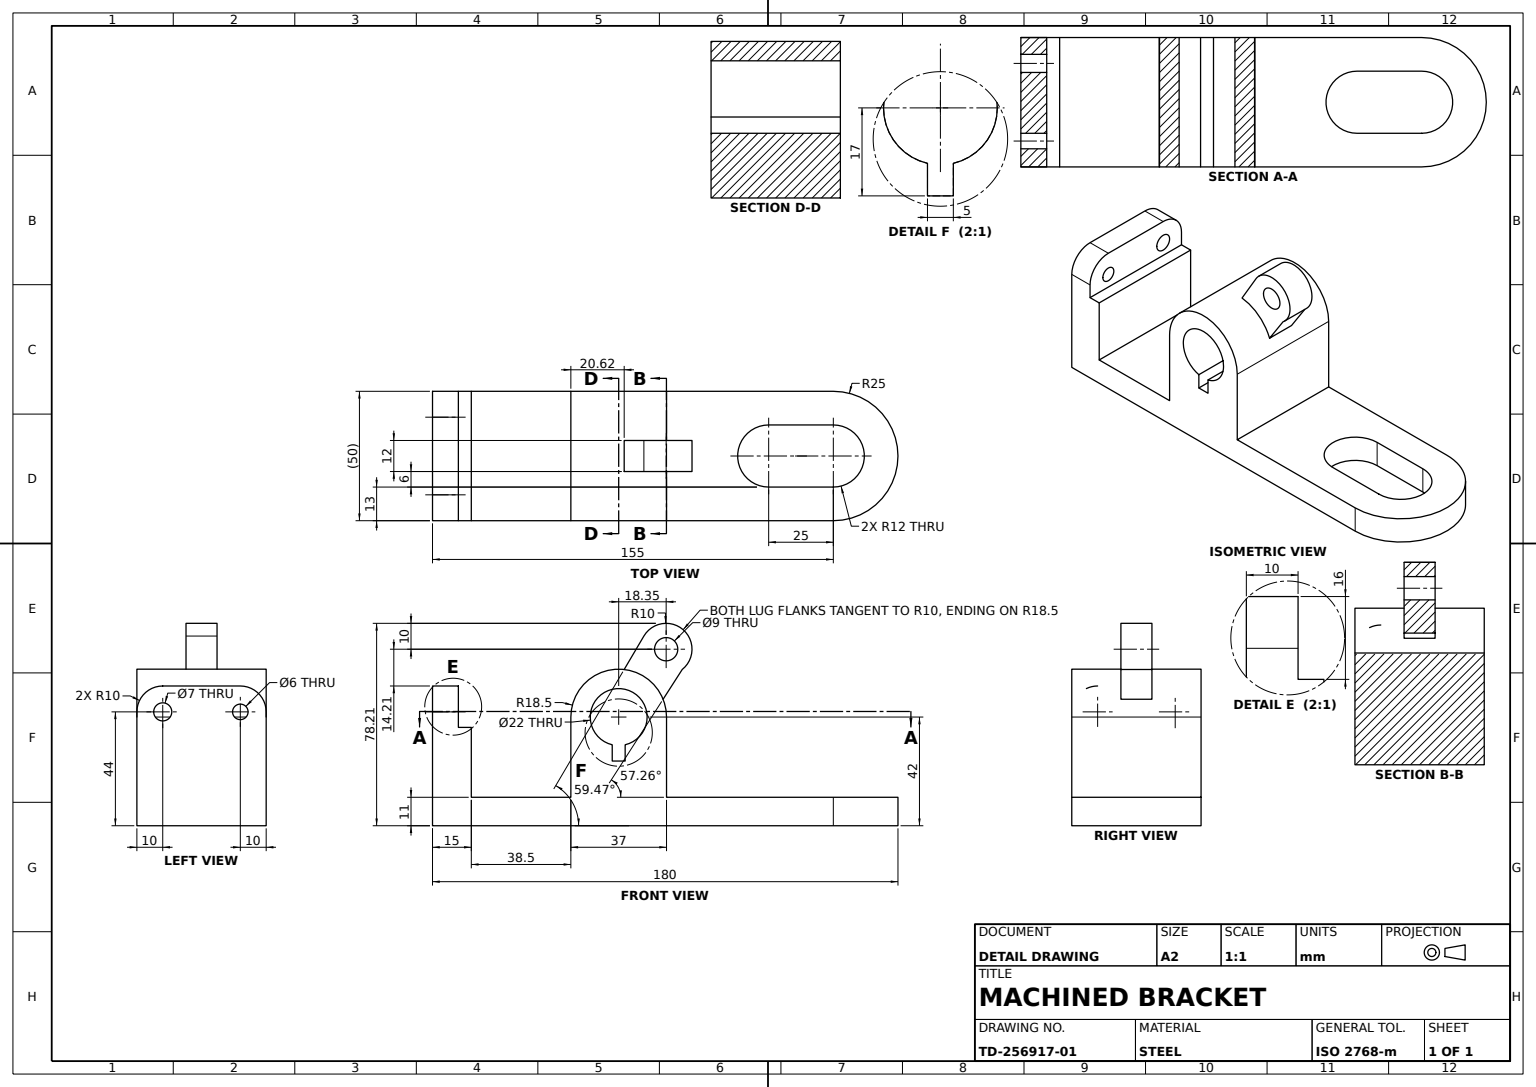
from build123d import *

# Parameters (mm, degrees)
BASE_PLATE_11MM_DEPTH    = 11
UPRIGHT_BLOCK_DEPTH      = 50
CHANNEL_CUT_DEPTH        = 50
FRONT_WALL_12MM_DEPTH    = 6
WALL_HOLE_SKETCH_R       = 4.5
WALL_THROUGH_HOLE_DEPTH  = 69
BORE_KEYWAY_CUT_DEPTH    = 69
HOUSING_PAD_SKETCH_W     = 15
HOUSING_PAD_SKETCH_H     = 50
HOUSING_PAD_DEPTH        = 27
BORE_HOUSING_SKETCH_W    = 10
BORE_HOUSING_SKETCH_H    = 16
BORE_HOUSING_DEPTH       = 50
HOUSING_FILLET_R10_A_R   = 10
HOUSING_FILLET_R10_B_R   = 10
CROSS_HOLE_SKETCH_R      = 3.5
CROSS_HOLE_SKETCH_R_2    = 3
HOUSING_CROSS_HOLE_DEPTH = 40


with BuildPart() as part:
    # Base Plate Sketch → Base Plate 11mm (new body)
    with BuildSketch(Plane(origin=(0, 0, 0), x_dir=(1, 0, 0), z_dir=(0, 1, 0))):
        with BuildLine():
            Line((-77.5, 25), (-77.5, -25))
            Line((-77.5, -25), (77.5, -25))
            ThreePointArc((77.5, -25), (102.5, 0), (77.5, 25))
            Line((77.5, 25), (-77.5, 25))
        make_face()
    extrude(amount=BASE_PLATE_11MM_DEPTH)

    # Upright Block Sketch → Upright Block (add)
    with BuildSketch(Plane.XY.offset(25)):
        with BuildLine():
            ThreePointArc((13, 42), (-5.5, 60.5), (-24, 42))
            Line((-24, 42), (-24, 11))
            Line((-24, 11), (13, 11))
            Line((13, 11), (13, 42))
        make_face()
    extrude(amount=-UPRIGHT_BLOCK_DEPTH)

    # Channel Cut Sketch → Channel Cut (cut)
    with BuildSketch(Plane.XY.offset(25)):
        with BuildLine():
            Line((-5.5, 25), (-8, 25))
            Line((-8, 25), (-8, 31.287857357))
            ThreePointArc((-8, 31.287857357), (-5.5, 53), (-3, 31.287857357))
            Line((-3, 31.287857357), (-3, 25))
            Line((-3, 25), (-5.5, 25))
        make_face()
    extrude(amount=-CHANNEL_CUT_DEPTH, mode=Mode.SUBTRACT)

    # Front Wall Sketch → Front Wall 12mm (add, symmetric)
    with BuildSketch(Plane.XY):
        with BuildLine():
            Line((4.241132249, 73.293301112), (-3.376902326, 60.37777071))
            Line((-3.376902326, 60.37777071), (11.674130016, 48.877445616))
            Line((11.674130016, 48.877445616), (19.069800109, 60.379004757))
            ThreePointArc((19.069800109, 60.379004757), (19.421965671, 75.753931979), (4.241132249, 73.293301112))
        make_face()
    extrude(amount=FRONT_WALL_12MM_DEPTH, both=True)

    # Wall Hole Sketch → Wall Through Hole (cut)
    with BuildSketch(Plane.XY.offset(6)):
        with Locations((12.854445963, 68.212865417)):
            Circle(WALL_HOLE_SKETCH_R)
    extrude(amount=-WALL_THROUGH_HOLE_DEPTH, mode=Mode.SUBTRACT)

    # Bore Keyway Sketch → Bore Keyway Cut (cut)
    with BuildSketch(Plane(origin=(0, 11, 0), x_dir=(1, 0, 0), z_dir=(0, 1, 0))):
        with BuildLine():
            Line((52.5, 12), (77.5, 12))
            ThreePointArc((77.5, 12), (89.5, 0), (77.5, -12))
            Line((77.5, -12), (52.5, -12))
            ThreePointArc((52.5, -12), (40.5, 0), (52.5, 12))
        make_face()
    extrude(amount=-BORE_KEYWAY_CUT_DEPTH, mode=Mode.SUBTRACT)

    # Housing Pad Sketch → Housing Pad (add)
    with BuildSketch(Plane(origin=(0, 11, 0), x_dir=(1, 0, 0), z_dir=(0, 1, 0))):
        with Locations((-70, 0)):
            Rectangle(HOUSING_PAD_SKETCH_W, HOUSING_PAD_SKETCH_H)
    extrude(amount=HOUSING_PAD_DEPTH)

    # Bore Housing Sketch → Bore Housing (add)
    with BuildSketch(Plane.XY.offset(25)):
        with Locations((-72.5, 46)):
            Rectangle(BORE_HOUSING_SKETCH_W, BORE_HOUSING_SKETCH_H)
    extrude(amount=-BORE_HOUSING_DEPTH)

    # Housing Fillet R10 A
    housing_fillet_r10_a_edges = [part.edges().sort_by_distance(p)[0] for p in [
        (-72.5, 54, 25),
    ]]
    fillet(housing_fillet_r10_a_edges, radius=HOUSING_FILLET_R10_A_R)

    # Housing Fillet R10 B
    housing_fillet_r10_b_edges = [part.edges().sort_by_distance(p)[0] for p in [
        (-72.5, 54, -25),
    ]]
    fillet(housing_fillet_r10_b_edges, radius=HOUSING_FILLET_R10_B_R)

    # Cross Hole Sketch → Housing Cross Hole (cut)
    with BuildSketch(Plane.ZY.offset(77.5)):
        with Locations((-15, 44)):
            Circle(CROSS_HOLE_SKETCH_R)
        with Locations((15, 44)):
            Circle(CROSS_HOLE_SKETCH_R_2)
    extrude(amount=-HOUSING_CROSS_HOLE_DEPTH, mode=Mode.SUBTRACT)


solid = part.part
